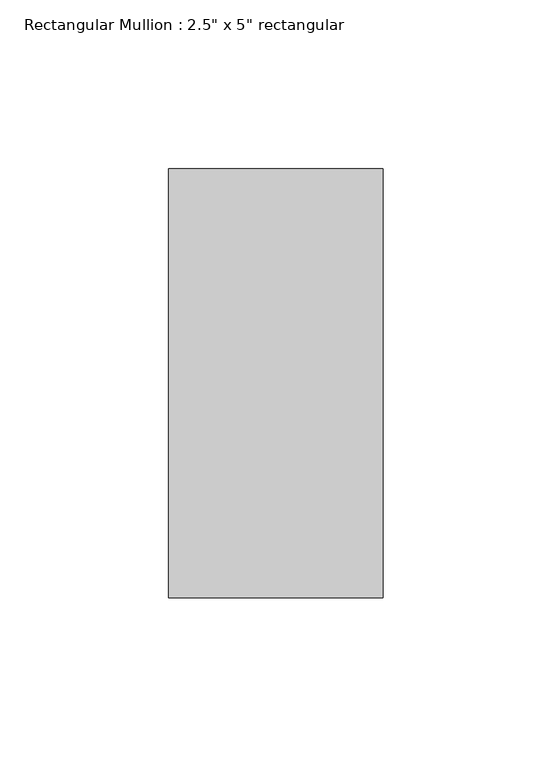
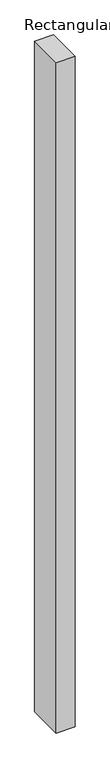
"""IFC4 building model written with IfcOpenShell, lengths in millimetres: member geometry."""

from ifc_helpers import new_model, si_unit, frame, origin, place, context, project, spatial, polyline, outline, extrude, source, transform, mapped, element, save


def member_5fae7eaf(model_context):
    return source(origin(), model_context, "Body", "SweptSolid", [
        extrude(outline(polyline([(31.75, 63.5), (31.75, -63.5), (-31.75, -63.5), (-31.75, 63.5), (31.75, 63.5)])), frame((0.0, 0.0, -2411.5809615), z_axis=(0.0, 0.0, 1.0), x_axis=(1.0, 0.0, 0.0)), (0.0, 0.0, 1.0), 2411.5809615),
    ])


if __name__ == "__main__":
    model = new_model("IFC4")
    model_context = context("Model", 3, world=origin())
    ifc_project = project(units=[si_unit("LENGTHUNIT", "METRE", prefix="MILLI")], contexts=[model_context])
    site = spatial("IfcSite", under=ifc_project)
    building = spatial("IfcBuilding", under=site)
    placement = place(None, origin())
    member_shape = member_5fae7eaf(model_context)
    element("IfcMember", 1, ObjectType="Rectangular Mullion : 2.5\" x 5\" rectangular", at=placement, inside=building, context=model_context, shape_type="MappedRepresentation", body=[
        mapped(member_shape, transform((0.0, 0.0, 0.0), x_axis=(1.0, 0.0, 0.0), y_axis=(0.0, 1.0, 0.0), z_axis=(0.0, 0.0, 1.0))),
    ])
    save(model, "model.ifc")

# Revit data of these elements
# Type "Rectangular Mullion : 2.5\" x 5\" rectangular"
#   built-in parameter 1007304 = 0.416667 (stored number, unit not read)
#   built-in parameter 1007301 = 0.104167 (stored number, unit not read)
#   built-in parameter 1007300 = 0.104167 (stored number, unit not read)
# Element 1 (IfcMember, "Rectangular Mullion : 2.5\" x 5\" rectangular")
#   Materials on its faces: "Aluminum"
# Materials
#   "Aluminum": class "Metal", colour RGB 247 247 247, transparency 0, Description = "Aluminum 6061", Cost = 0
